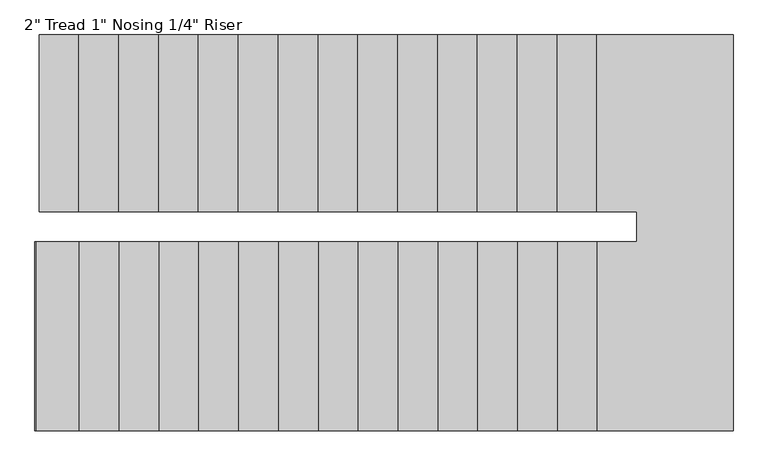
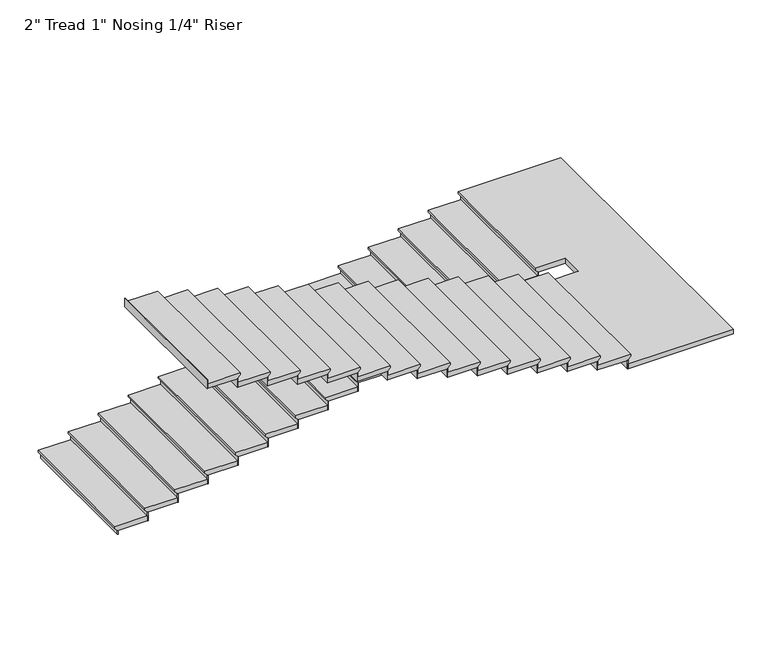
"""IFC4 building model written with IfcOpenShell, lengths in millimetres: stair flight geometry."""

from ifc_helpers import new_model, si_unit, origin, place, context, project, spatial, faceted_brep, source, transform, mapped, element, save


def stair_flight_f9fdc227(model_context):
    return source(origin(), model_context, "Body", "Brep", [
        faceted_brep([(-5254.0891351, 11154.2082924, 72.39), (-5254.0891351, 11154.2082924, 91.44), (-5254.0891351, 12506.0715905, 91.44), (-5254.0891351, 12506.0715905, 72.39), (-5228.6891351, 11154.2082924, 46.99), (-5228.6891351, 12506.0715905, 46.99), (-4923.8891351, 11154.2082924, 91.44), (-4923.8891351, 12506.0715905, 91.44), (-5228.6891351, 12506.0715905, 40.64), (-4923.8891351, 12506.0715905, 40.64), (-4923.8891351, 11154.2082924, 40.64), (-5228.6891351, 11154.2082924, 40.64)], [[[0, 1, 2, 3]], [[4, 0, 3, 5]], [[2, 1, 6, 7]], [[8, 9, 10, 11]], [[2, 7, 9, 8, 5, 3]], [[8, 11, 4, 5]], [[6, 1, 0, 4, 11, 10]], [[7, 6, 10, 9]]]),
        faceted_brep([(-5228.6891351, 11154.2082924, 40.64), (-5228.6891351, 11154.2082924, 0.0), (-5222.3391351, 11154.2082924, 0.0), (-5222.3391351, 11154.2082924, 40.64), (-5228.6891351, 12506.0715905, 40.64), (-5222.3391351, 12506.0715905, 40.64), (-5222.3391351, 12506.0715905, 0.0), (-5228.6891351, 12506.0715905, 0.0)], [[[0, 1, 2, 3]], [[4, 5, 6, 7]], [[1, 0, 4, 7]], [[2, 1, 7, 6]], [[3, 2, 6, 5]], [[0, 3, 5, 4]]]),
        faceted_brep([(-4923.8891351, 11154.2082924, 132.08), (-4923.8891351, 11154.2082924, 40.64), (-4917.5391351, 11154.2082924, 40.64), (-4917.5391351, 11154.2082924, 132.08), (-4923.8891351, 12506.0715905, 132.08), (-4917.5391351, 12506.0715905, 132.08), (-4917.5391351, 12506.0715905, 40.64), (-4923.8891351, 12506.0715905, 40.64)], [[[0, 1, 2, 3]], [[4, 5, 6, 7]], [[1, 0, 4, 7]], [[2, 1, 7, 6]], [[3, 2, 6, 5]], [[0, 3, 5, 4]]]),
        faceted_brep([(-4949.2891351, 12506.0715905, 182.88), (-4949.2891351, 11154.2082924, 182.88), (-4619.0891351, 11154.2082924, 182.88), (-4619.0891351, 12506.0715905, 182.88), (-4923.8891351, 12506.0715905, 132.08), (-4619.0891351, 12506.0715905, 132.08), (-4619.0891351, 11154.2082924, 132.08), (-4923.8891351, 11154.2082924, 132.08), (-4923.8891351, 12506.0715905, 138.43), (-4949.2891351, 12506.0715905, 163.83), (-4923.8891351, 11154.2082924, 138.43), (-4949.2891351, 11154.2082924, 163.83)], [[[0, 1, 2, 3]], [[4, 5, 6, 7]], [[0, 3, 5, 4, 8, 9]], [[4, 7, 10, 8]], [[2, 1, 11, 10, 7, 6]], [[3, 2, 6, 5]], [[11, 1, 0, 9]], [[10, 11, 9, 8]]]),
        faceted_brep([(-4619.0891351, 11154.2082924, 223.52), (-4619.0891351, 11154.2082924, 132.08), (-4612.7391351, 11154.2082924, 132.08), (-4612.7391351, 11154.2082924, 223.52), (-4619.0891351, 12506.0715905, 223.52), (-4612.7391351, 12506.0715905, 223.52), (-4612.7391351, 12506.0715905, 132.08), (-4619.0891351, 12506.0715905, 132.08)], [[[0, 1, 2, 3]], [[4, 5, 6, 7]], [[1, 0, 4, 7]], [[2, 1, 7, 6]], [[3, 2, 6, 5]], [[0, 3, 5, 4]]]),
        faceted_brep([(-4644.4891351, 12506.0715905, 274.32), (-4644.4891351, 11154.2082924, 274.32), (-4314.2891351, 11154.2082924, 274.32), (-4314.2891351, 12506.0715905, 274.32), (-4619.0891351, 12506.0715905, 223.52), (-4314.2891351, 12506.0715905, 223.52), (-4314.2891351, 11154.2082924, 223.52), (-4619.0891351, 11154.2082924, 223.52), (-4619.0891351, 12506.0715905, 229.87), (-4644.4891351, 12506.0715905, 255.27), (-4619.0891351, 11154.2082924, 229.87), (-4644.4891351, 11154.2082924, 255.27)], [[[0, 1, 2, 3]], [[4, 5, 6, 7]], [[0, 3, 5, 4, 8, 9]], [[4, 7, 10, 8]], [[2, 1, 11, 10, 7, 6]], [[3, 2, 6, 5]], [[11, 1, 0, 9]], [[10, 11, 9, 8]]]),
        faceted_brep([(-4314.2891351, 11154.2082924, 314.96), (-4314.2891351, 11154.2082924, 223.52), (-4307.9391351, 11154.2082924, 223.52), (-4307.9391351, 11154.2082924, 314.96), (-4314.2891351, 12506.0715905, 314.96), (-4307.9391351, 12506.0715905, 314.96), (-4307.9391351, 12506.0715905, 223.52), (-4314.2891351, 12506.0715905, 223.52)], [[[0, 1, 2, 3]], [[4, 5, 6, 7]], [[1, 0, 4, 7]], [[2, 1, 7, 6]], [[3, 2, 6, 5]], [[0, 3, 5, 4]]]),
        faceted_brep([(-4339.6891351, 12506.0715905, 365.76), (-4339.6891351, 11154.2082924, 365.76), (-4009.4891351, 11154.2082924, 365.76), (-4009.4891351, 12506.0715905, 365.76), (-4314.2891351, 12506.0715905, 314.96), (-4009.4891351, 12506.0715905, 314.96), (-4009.4891351, 11154.2082924, 314.96), (-4314.2891351, 11154.2082924, 314.96), (-4314.2891351, 12506.0715905, 321.31), (-4339.6891351, 12506.0715905, 346.71), (-4314.2891351, 11154.2082924, 321.31), (-4339.6891351, 11154.2082924, 346.71)], [[[0, 1, 2, 3]], [[4, 5, 6, 7]], [[0, 3, 5, 4, 8, 9]], [[4, 7, 10, 8]], [[2, 1, 11, 10, 7, 6]], [[3, 2, 6, 5]], [[11, 1, 0, 9]], [[10, 11, 9, 8]]]),
        faceted_brep([(-4009.4891351, 11154.2082924, 406.4), (-4009.4891351, 11154.2082924, 314.96), (-4003.1391351, 11154.2082924, 314.96), (-4003.1391351, 11154.2082924, 406.4), (-4009.4891351, 12506.0715905, 406.4), (-4003.1391351, 12506.0715905, 406.4), (-4003.1391351, 12506.0715905, 314.96), (-4009.4891351, 12506.0715905, 314.96)], [[[0, 1, 2, 3]], [[4, 5, 6, 7]], [[1, 0, 4, 7]], [[2, 1, 7, 6]], [[3, 2, 6, 5]], [[0, 3, 5, 4]]]),
        faceted_brep([(-4034.8891351, 12506.0715905, 457.2), (-4034.8891351, 11154.2082924, 457.2), (-3704.6891351, 11154.2082924, 457.2), (-3704.6891351, 12506.0715905, 457.2), (-4009.4891351, 12506.0715905, 406.4), (-3704.6891351, 12506.0715905, 406.4), (-3704.6891351, 11154.2082924, 406.4), (-4009.4891351, 11154.2082924, 406.4), (-4009.4891351, 12506.0715905, 412.75), (-4034.8891351, 12506.0715905, 438.15), (-4009.4891351, 11154.2082924, 412.75), (-4034.8891351, 11154.2082924, 438.15)], [[[0, 1, 2, 3]], [[4, 5, 6, 7]], [[0, 3, 5, 4, 8, 9]], [[4, 7, 10, 8]], [[2, 1, 11, 10, 7, 6]], [[3, 2, 6, 5]], [[11, 1, 0, 9]], [[10, 11, 9, 8]]]),
        faceted_brep([(-3704.6891351, 11154.2082924, 497.84), (-3704.6891351, 11154.2082924, 406.4), (-3698.3391351, 11154.2082924, 406.4), (-3698.3391351, 11154.2082924, 497.84), (-3704.6891351, 12506.0715905, 497.84), (-3698.3391351, 12506.0715905, 497.84), (-3698.3391351, 12506.0715905, 406.4), (-3704.6891351, 12506.0715905, 406.4)], [[[0, 1, 2, 3]], [[4, 5, 6, 7]], [[1, 0, 4, 7]], [[2, 1, 7, 6]], [[3, 2, 6, 5]], [[0, 3, 5, 4]]]),
        faceted_brep([(-3730.0891351, 12506.0715905, 548.64), (-3730.0891351, 11154.2082924, 548.64), (-3399.8891351, 11154.2082924, 548.64), (-3399.8891351, 12506.0715905, 548.64), (-3704.6891351, 12506.0715905, 497.84), (-3399.8891351, 12506.0715905, 497.84), (-3399.8891351, 11154.2082924, 497.84), (-3704.6891351, 11154.2082924, 497.84), (-3704.6891351, 12506.0715905, 504.19), (-3730.0891351, 12506.0715905, 529.59), (-3704.6891351, 11154.2082924, 504.19), (-3730.0891351, 11154.2082924, 529.59)], [[[0, 1, 2, 3]], [[4, 5, 6, 7]], [[0, 3, 5, 4, 8, 9]], [[4, 7, 10, 8]], [[2, 1, 11, 10, 7, 6]], [[3, 2, 6, 5]], [[11, 1, 0, 9]], [[10, 11, 9, 8]]]),
        faceted_brep([(-3399.8891351, 11154.2082924, 589.28), (-3399.8891351, 11154.2082924, 497.84), (-3393.5391351, 11154.2082924, 497.84), (-3393.5391351, 11154.2082924, 589.28), (-3399.8891351, 12506.0715905, 589.28), (-3393.5391351, 12506.0715905, 589.28), (-3393.5391351, 12506.0715905, 497.84), (-3399.8891351, 12506.0715905, 497.84)], [[[0, 1, 2, 3]], [[4, 5, 6, 7]], [[1, 0, 4, 7]], [[2, 1, 7, 6]], [[3, 2, 6, 5]], [[0, 3, 5, 4]]]),
        faceted_brep([(-3425.2891351, 12506.0715905, 640.08), (-3425.2891351, 11154.2082924, 640.08), (-3095.0891351, 11154.2082924, 640.08), (-3095.0891351, 12506.0715905, 640.08), (-3399.8891351, 12506.0715905, 589.28), (-3095.0891351, 12506.0715905, 589.28), (-3095.0891351, 11154.2082924, 589.28), (-3399.8891351, 11154.2082924, 589.28), (-3399.8891351, 12506.0715905, 595.63), (-3425.2891351, 12506.0715905, 621.03), (-3399.8891351, 11154.2082924, 595.63), (-3425.2891351, 11154.2082924, 621.03)], [[[0, 1, 2, 3]], [[4, 5, 6, 7]], [[0, 3, 5, 4, 8, 9]], [[4, 7, 10, 8]], [[2, 1, 11, 10, 7, 6]], [[3, 2, 6, 5]], [[11, 1, 0, 9]], [[10, 11, 9, 8]]]),
        faceted_brep([(-3095.0891351, 11154.2082924, 680.72), (-3095.0891351, 11154.2082924, 589.28), (-3088.7391351, 11154.2082924, 589.28), (-3088.7391351, 11154.2082924, 680.72), (-3095.0891351, 12506.0715905, 680.72), (-3088.7391351, 12506.0715905, 680.72), (-3088.7391351, 12506.0715905, 589.28), (-3095.0891351, 12506.0715905, 589.28)], [[[0, 1, 2, 3]], [[4, 5, 6, 7]], [[1, 0, 4, 7]], [[2, 1, 7, 6]], [[3, 2, 6, 5]], [[0, 3, 5, 4]]]),
        faceted_brep([(-3120.4891351, 12506.0715905, 731.52), (-3120.4891351, 11154.2082924, 731.52), (-2790.2891351, 11154.2082924, 731.52), (-2790.2891351, 12506.0715905, 731.52), (-3095.0891351, 12506.0715905, 680.72), (-2790.2891351, 12506.0715905, 680.72), (-2790.2891351, 11154.2082924, 680.72), (-3095.0891351, 11154.2082924, 680.72), (-3095.0891351, 12506.0715905, 687.07), (-3120.4891351, 12506.0715905, 712.47), (-3095.0891351, 11154.2082924, 687.07), (-3120.4891351, 11154.2082924, 712.47)], [[[0, 1, 2, 3]], [[4, 5, 6, 7]], [[0, 3, 5, 4, 8, 9]], [[4, 7, 10, 8]], [[2, 1, 11, 10, 7, 6]], [[3, 2, 6, 5]], [[11, 1, 0, 9]], [[10, 11, 9, 8]]]),
        faceted_brep([(-2790.2891351, 11154.2082924, 772.16), (-2790.2891351, 11154.2082924, 680.72), (-2783.9391351, 11154.2082924, 680.72), (-2783.9391351, 11154.2082924, 772.16), (-2790.2891351, 12506.0715905, 772.16), (-2783.9391351, 12506.0715905, 772.16), (-2783.9391351, 12506.0715905, 680.72), (-2790.2891351, 12506.0715905, 680.72)], [[[0, 1, 2, 3]], [[4, 5, 6, 7]], [[1, 0, 4, 7]], [[2, 1, 7, 6]], [[3, 2, 6, 5]], [[0, 3, 5, 4]]]),
        faceted_brep([(-2815.6891351, 12506.0715905, 822.96), (-2815.6891351, 11154.2082924, 822.96), (-2485.4891351, 11154.2082924, 822.96), (-2485.4891351, 12506.0715905, 822.96), (-2790.2891351, 12506.0715905, 772.16), (-2485.4891351, 12506.0715905, 772.16), (-2485.4891351, 11154.2082924, 772.16), (-2790.2891351, 11154.2082924, 772.16), (-2790.2891351, 12506.0715905, 778.51), (-2815.6891351, 12506.0715905, 803.91), (-2790.2891351, 11154.2082924, 778.51), (-2815.6891351, 11154.2082924, 803.91)], [[[0, 1, 2, 3]], [[4, 5, 6, 7]], [[0, 3, 5, 4, 8, 9]], [[4, 7, 10, 8]], [[2, 1, 11, 10, 7, 6]], [[3, 2, 6, 5]], [[11, 1, 0, 9]], [[10, 11, 9, 8]]]),
        faceted_brep([(-2485.4891351, 11154.2082924, 863.6), (-2485.4891351, 11154.2082924, 772.16), (-2479.1391351, 11154.2082924, 772.16), (-2479.1391351, 11154.2082924, 863.6), (-2485.4891351, 12506.0715905, 863.6), (-2479.1391351, 12506.0715905, 863.6), (-2479.1391351, 12506.0715905, 772.16), (-2485.4891351, 12506.0715905, 772.16)], [[[0, 1, 2, 3]], [[4, 5, 6, 7]], [[1, 0, 4, 7]], [[2, 1, 7, 6]], [[3, 2, 6, 5]], [[0, 3, 5, 4]]]),
        faceted_brep([(-2510.8891351, 12506.0715905, 914.4), (-2510.8891351, 11154.2082924, 914.4), (-2180.6891351, 11154.2082924, 914.4), (-2180.6891351, 12506.0715905, 914.4), (-2485.4891351, 12506.0715905, 863.6), (-2180.6891351, 12506.0715905, 863.6), (-2180.6891351, 11154.2082924, 863.6), (-2485.4891351, 11154.2082924, 863.6), (-2485.4891351, 12506.0715905, 869.95), (-2510.8891351, 12506.0715905, 895.35), (-2485.4891351, 11154.2082924, 869.95), (-2510.8891351, 11154.2082924, 895.35)], [[[0, 1, 2, 3]], [[4, 5, 6, 7]], [[0, 3, 5, 4, 8, 9]], [[4, 7, 10, 8]], [[2, 1, 11, 10, 7, 6]], [[3, 2, 6, 5]], [[11, 1, 0, 9]], [[10, 11, 9, 8]]]),
        faceted_brep([(-2180.6891351, 11154.2082924, 955.04), (-2180.6891351, 11154.2082924, 863.6), (-2174.3391351, 11154.2082924, 863.6), (-2174.3391351, 11154.2082924, 955.04), (-2180.6891351, 12506.0715905, 955.04), (-2174.3391351, 12506.0715905, 955.04), (-2174.3391351, 12506.0715905, 863.6), (-2180.6891351, 12506.0715905, 863.6)], [[[0, 1, 2, 3]], [[4, 5, 6, 7]], [[1, 0, 4, 7]], [[2, 1, 7, 6]], [[3, 2, 6, 5]], [[0, 3, 5, 4]]]),
        faceted_brep([(-2206.0891351, 12506.0715905, 1005.84), (-2206.0891351, 11154.2082924, 1005.84), (-1875.8891351, 11154.2082924, 1005.84), (-1875.8891351, 12506.0715905, 1005.84), (-2180.6891351, 12506.0715905, 955.04), (-1875.8891351, 12506.0715905, 955.04), (-1875.8891351, 11154.2082924, 955.04), (-2180.6891351, 11154.2082924, 955.04), (-2180.6891351, 12506.0715905, 961.39), (-2206.0891351, 12506.0715905, 986.79), (-2180.6891351, 11154.2082924, 961.39), (-2206.0891351, 11154.2082924, 986.79)], [[[0, 1, 2, 3]], [[4, 5, 6, 7]], [[0, 3, 5, 4, 8, 9]], [[4, 7, 10, 8]], [[2, 1, 11, 10, 7, 6]], [[3, 2, 6, 5]], [[11, 1, 0, 9]], [[10, 11, 9, 8]]]),
        faceted_brep([(-1875.8891351, 11154.2082924, 1046.48), (-1875.8891351, 11154.2082924, 955.04), (-1869.5391351, 11154.2082924, 955.04), (-1869.5391351, 11154.2082924, 1046.48), (-1875.8891351, 12506.0715905, 1046.48), (-1869.5391351, 12506.0715905, 1046.48), (-1869.5391351, 12506.0715905, 955.04), (-1875.8891351, 12506.0715905, 955.04)], [[[0, 1, 2, 3]], [[4, 5, 6, 7]], [[1, 0, 4, 7]], [[2, 1, 7, 6]], [[3, 2, 6, 5]], [[0, 3, 5, 4]]]),
        faceted_brep([(-1901.2891351, 12506.0715905, 1097.28), (-1901.2891351, 11154.2082924, 1097.28), (-1571.0891351, 11154.2082924, 1097.28), (-1571.0891351, 12506.0715905, 1097.28), (-1875.8891351, 12506.0715905, 1046.48), (-1571.0891351, 12506.0715905, 1046.48), (-1571.0891351, 11154.2082924, 1046.48), (-1875.8891351, 11154.2082924, 1046.48), (-1875.8891351, 12506.0715905, 1052.83), (-1901.2891351, 12506.0715905, 1078.23), (-1875.8891351, 11154.2082924, 1052.83), (-1901.2891351, 11154.2082924, 1078.23)], [[[0, 1, 2, 3]], [[4, 5, 6, 7]], [[0, 3, 5, 4, 8, 9]], [[4, 7, 10, 8]], [[2, 1, 11, 10, 7, 6]], [[3, 2, 6, 5]], [[11, 1, 0, 9]], [[10, 11, 9, 8]]]),
        faceted_brep([(-1571.0891351, 11154.2082924, 1137.92), (-1571.0891351, 11154.2082924, 1046.48), (-1564.7391351, 11154.2082924, 1046.48), (-1564.7391351, 11154.2082924, 1137.92), (-1571.0891351, 12506.0715905, 1137.92), (-1564.7391351, 12506.0715905, 1137.92), (-1564.7391351, 12506.0715905, 1046.48), (-1571.0891351, 12506.0715905, 1046.48)], [[[0, 1, 2, 3]], [[4, 5, 6, 7]], [[1, 0, 4, 7]], [[2, 1, 7, 6]], [[3, 2, 6, 5]], [[0, 3, 5, 4]]]),
        faceted_brep([(-1596.4891351, 12506.0715905, 1188.72), (-1596.4891351, 11154.2082924, 1188.72), (-1266.2891351, 11154.2082924, 1188.72), (-1266.2891351, 12506.0715905, 1188.72), (-1571.0891351, 12506.0715905, 1137.92), (-1266.2891351, 12506.0715905, 1137.92), (-1266.2891351, 11154.2082924, 1137.92), (-1571.0891351, 11154.2082924, 1137.92), (-1571.0891351, 12506.0715905, 1144.27), (-1596.4891351, 12506.0715905, 1169.67), (-1571.0891351, 11154.2082924, 1144.27), (-1596.4891351, 11154.2082924, 1169.67)], [[[0, 1, 2, 3]], [[4, 5, 6, 7]], [[0, 3, 5, 4, 8, 9]], [[4, 7, 10, 8]], [[2, 1, 11, 10, 7, 6]], [[3, 2, 6, 5]], [[11, 1, 0, 9]], [[10, 11, 9, 8]]]),
        faceted_brep([(-1266.2891351, 11154.2082924, 1229.36), (-1266.2891351, 11154.2082924, 1137.92), (-1259.9391351, 11154.2082924, 1137.92), (-1259.9391351, 11154.2082924, 1229.36), (-1266.2891351, 12506.0715905, 1229.36), (-1259.9391351, 12506.0715905, 1229.36), (-1259.9391351, 12506.0715905, 1137.92), (-1266.2891351, 12506.0715905, 1137.92)], [[[0, 1, 2, 3]], [[4, 5, 6, 7]], [[1, 0, 4, 7]], [[2, 1, 7, 6]], [[3, 2, 6, 5]], [[0, 3, 5, 4]]]),
        faceted_brep([(-1291.6891351, 12506.0715905, 1280.16), (-1291.6891351, 11154.2082924, 1280.16), (-961.4891351, 11154.2082924, 1280.16), (-961.4891351, 12506.0715905, 1280.16), (-1266.2891351, 12506.0715905, 1229.36), (-961.4891351, 12506.0715905, 1229.36), (-961.4891351, 11154.2082924, 1229.36), (-1266.2891351, 11154.2082924, 1229.36), (-1266.2891351, 12506.0715905, 1235.71), (-1291.6891351, 12506.0715905, 1261.11), (-1266.2891351, 11154.2082924, 1235.71), (-1291.6891351, 11154.2082924, 1261.11)], [[[0, 1, 2, 3]], [[4, 5, 6, 7]], [[0, 3, 5, 4, 8, 9]], [[4, 7, 10, 8]], [[2, 1, 11, 10, 7, 6]], [[3, 2, 6, 5]], [[11, 1, 0, 9]], [[10, 11, 9, 8]]]),
        faceted_brep([(-961.4891351, 11154.2082924, 1320.8), (-961.4891351, 11154.2082924, 1229.36), (-955.1391351, 11154.2082924, 1229.36), (-955.1391351, 11154.2082924, 1320.8), (-961.4891351, 12506.0715905, 1320.8), (-955.1391351, 12506.0715905, 1320.8), (-955.1391351, 12506.0715905, 1229.36), (-961.4891351, 12506.0715905, 1229.36)], [[[0, 1, 2, 3]], [[4, 5, 6, 7]], [[1, 0, 4, 7]], [[2, 1, 7, 6]], [[3, 2, 6, 5]], [[0, 3, 5, 4]]]),
        faceted_brep([(-1012.2891351, 9478.4949943, 1371.6), (54.5108649, 9478.4949943, 1371.6), (54.5108649, 12506.0715905, 1371.6), (-986.8891351, 12506.0715905, 1371.6), (-986.8891351, 11154.2082924, 1371.6), (-682.0891351, 11154.2082924, 1371.6), (-682.0891351, 10925.6082924, 1371.6), (-1012.2891351, 10925.6082924, 1371.6), (54.5108649, 9478.4949943, 1320.8), (-1012.2891351, 9478.4949943, 1320.8), (-1012.2891351, 10925.6082924, 1320.8), (-682.0891351, 10925.6082924, 1320.8), (-682.0891351, 11154.2082924, 1320.8), (-961.4891351, 11154.2082924, 1320.8), (-961.4891351, 12506.0715905, 1320.8), (54.5108649, 12506.0715905, 1320.8), (-961.4891351, 12506.0715905, 1327.15), (-986.8891351, 12506.0715905, 1352.55), (-961.4891351, 11154.2082924, 1327.15), (-986.8891351, 11154.2082924, 1352.55)], [[[0, 1, 2, 3, 4, 5, 6, 7]], [[8, 9, 10, 11, 12, 13, 14, 15]], [[1, 0, 9, 8]], [[2, 1, 8, 15]], [[3, 2, 15, 14, 16, 17]], [[14, 13, 18, 16]], [[5, 4, 19, 18, 13, 12]], [[6, 5, 12, 11]], [[7, 6, 11, 10]], [[0, 7, 10, 9]], [[19, 4, 3, 17]], [[18, 19, 17, 16]]]),
        faceted_brep([(-1012.2891351, 10925.6082924, 1412.24), (-1012.2891351, 10925.6082924, 1320.8), (-1018.6391351, 10925.6082924, 1320.8), (-1018.6391351, 10925.6082924, 1412.24), (-1012.2891351, 9478.4949943, 1412.24), (-1018.6391351, 9478.4949943, 1412.24), (-1018.6391351, 9478.4949943, 1320.8), (-1012.2891351, 9478.4949943, 1320.8)], [[[0, 1, 2, 3]], [[4, 5, 6, 7]], [[1, 0, 4, 7]], [[2, 1, 7, 6]], [[3, 2, 6, 5]], [[0, 3, 5, 4]]]),
        faceted_brep([(-986.8891351, 9478.4949943, 1463.04), (-986.8891351, 10925.6082924, 1463.04), (-1317.0891351, 10925.6082924, 1463.04), (-1317.0891351, 9478.4949943, 1463.04), (-1012.2891351, 9478.4949943, 1412.24), (-1317.0891351, 9478.4949943, 1412.24), (-1317.0891351, 10925.6082924, 1412.24), (-1012.2891351, 10925.6082924, 1412.24), (-1012.2891351, 9478.4949943, 1418.59), (-986.8891351, 9478.4949943, 1443.99), (-1012.2891351, 10925.6082924, 1418.59), (-986.8891351, 10925.6082924, 1443.99)], [[[0, 1, 2, 3]], [[4, 5, 6, 7]], [[0, 3, 5, 4, 8, 9]], [[4, 7, 10, 8]], [[2, 1, 11, 10, 7, 6]], [[3, 2, 6, 5]], [[11, 1, 0, 9]], [[10, 11, 9, 8]]]),
        faceted_brep([(-1317.0891351, 10925.6082924, 1503.68), (-1317.0891351, 10925.6082924, 1412.24), (-1323.4391351, 10925.6082924, 1412.24), (-1323.4391351, 10925.6082924, 1503.68), (-1317.0891351, 9478.4949943, 1503.68), (-1323.4391351, 9478.4949943, 1503.68), (-1323.4391351, 9478.4949943, 1412.24), (-1317.0891351, 9478.4949943, 1412.24)], [[[0, 1, 2, 3]], [[4, 5, 6, 7]], [[1, 0, 4, 7]], [[2, 1, 7, 6]], [[3, 2, 6, 5]], [[0, 3, 5, 4]]]),
        faceted_brep([(-1291.6891351, 9478.4949943, 1554.48), (-1291.6891351, 10925.6082924, 1554.48), (-1621.8891351, 10925.6082924, 1554.48), (-1621.8891351, 9478.4949943, 1554.48), (-1317.0891351, 9478.4949943, 1503.68), (-1621.8891351, 9478.4949943, 1503.68), (-1621.8891351, 10925.6082924, 1503.68), (-1317.0891351, 10925.6082924, 1503.68), (-1317.0891351, 9478.4949943, 1510.03), (-1291.6891351, 9478.4949943, 1535.43), (-1317.0891351, 10925.6082924, 1510.03), (-1291.6891351, 10925.6082924, 1535.43)], [[[0, 1, 2, 3]], [[4, 5, 6, 7]], [[0, 3, 5, 4, 8, 9]], [[4, 7, 10, 8]], [[2, 1, 11, 10, 7, 6]], [[3, 2, 6, 5]], [[11, 1, 0, 9]], [[10, 11, 9, 8]]]),
        faceted_brep([(-1621.8891351, 10925.6082924, 1595.12), (-1621.8891351, 10925.6082924, 1503.68), (-1628.2391351, 10925.6082924, 1503.68), (-1628.2391351, 10925.6082924, 1595.12), (-1621.8891351, 9478.4949943, 1595.12), (-1628.2391351, 9478.4949943, 1595.12), (-1628.2391351, 9478.4949943, 1503.68), (-1621.8891351, 9478.4949943, 1503.68)], [[[0, 1, 2, 3]], [[4, 5, 6, 7]], [[1, 0, 4, 7]], [[2, 1, 7, 6]], [[3, 2, 6, 5]], [[0, 3, 5, 4]]]),
        faceted_brep([(-1596.4891351, 9478.4949943, 1645.92), (-1596.4891351, 10925.6082924, 1645.92), (-1926.6891351, 10925.6082924, 1645.92), (-1926.6891351, 9478.4949943, 1645.92), (-1621.8891351, 9478.4949943, 1595.12), (-1926.6891351, 9478.4949943, 1595.12), (-1926.6891351, 10925.6082924, 1595.12), (-1621.8891351, 10925.6082924, 1595.12), (-1621.8891351, 9478.4949943, 1601.47), (-1596.4891351, 9478.4949943, 1626.87), (-1621.8891351, 10925.6082924, 1601.47), (-1596.4891351, 10925.6082924, 1626.87)], [[[0, 1, 2, 3]], [[4, 5, 6, 7]], [[0, 3, 5, 4, 8, 9]], [[4, 7, 10, 8]], [[2, 1, 11, 10, 7, 6]], [[3, 2, 6, 5]], [[11, 1, 0, 9]], [[10, 11, 9, 8]]]),
        faceted_brep([(-1926.6891351, 10925.6082924, 1686.56), (-1926.6891351, 10925.6082924, 1595.12), (-1933.0391351, 10925.6082924, 1595.12), (-1933.0391351, 10925.6082924, 1686.56), (-1926.6891351, 9478.4949943, 1686.56), (-1933.0391351, 9478.4949943, 1686.56), (-1933.0391351, 9478.4949943, 1595.12), (-1926.6891351, 9478.4949943, 1595.12)], [[[0, 1, 2, 3]], [[4, 5, 6, 7]], [[1, 0, 4, 7]], [[2, 1, 7, 6]], [[3, 2, 6, 5]], [[0, 3, 5, 4]]]),
        faceted_brep([(-1901.2891351, 9478.4949943, 1737.36), (-1901.2891351, 10925.6082924, 1737.36), (-2231.4891351, 10925.6082924, 1737.36), (-2231.4891351, 9478.4949943, 1737.36), (-1926.6891351, 9478.4949943, 1686.56), (-2231.4891351, 9478.4949943, 1686.56), (-2231.4891351, 10925.6082924, 1686.56), (-1926.6891351, 10925.6082924, 1686.56), (-1926.6891351, 9478.4949943, 1692.91), (-1901.2891351, 9478.4949943, 1718.31), (-1926.6891351, 10925.6082924, 1692.91), (-1901.2891351, 10925.6082924, 1718.31)], [[[0, 1, 2, 3]], [[4, 5, 6, 7]], [[0, 3, 5, 4, 8, 9]], [[4, 7, 10, 8]], [[2, 1, 11, 10, 7, 6]], [[3, 2, 6, 5]], [[11, 1, 0, 9]], [[10, 11, 9, 8]]]),
        faceted_brep([(-2231.4891351, 10925.6082924, 1778.0), (-2231.4891351, 10925.6082924, 1686.56), (-2237.8391351, 10925.6082924, 1686.56), (-2237.8391351, 10925.6082924, 1778.0), (-2231.4891351, 9478.4949943, 1778.0), (-2237.8391351, 9478.4949943, 1778.0), (-2237.8391351, 9478.4949943, 1686.56), (-2231.4891351, 9478.4949943, 1686.56)], [[[0, 1, 2, 3]], [[4, 5, 6, 7]], [[1, 0, 4, 7]], [[2, 1, 7, 6]], [[3, 2, 6, 5]], [[0, 3, 5, 4]]]),
        faceted_brep([(-2206.0891351, 9478.4949943, 1828.8), (-2206.0891351, 10925.6082924, 1828.8), (-2536.2891351, 10925.6082924, 1828.8), (-2536.2891351, 9478.4949943, 1828.8), (-2231.4891351, 9478.4949943, 1778.0), (-2536.2891351, 9478.4949943, 1778.0), (-2536.2891351, 10925.6082924, 1778.0), (-2231.4891351, 10925.6082924, 1778.0), (-2231.4891351, 9478.4949943, 1784.35), (-2206.0891351, 9478.4949943, 1809.75), (-2231.4891351, 10925.6082924, 1784.35), (-2206.0891351, 10925.6082924, 1809.75)], [[[0, 1, 2, 3]], [[4, 5, 6, 7]], [[0, 3, 5, 4, 8, 9]], [[4, 7, 10, 8]], [[2, 1, 11, 10, 7, 6]], [[3, 2, 6, 5]], [[11, 1, 0, 9]], [[10, 11, 9, 8]]]),
        faceted_brep([(-2536.2891351, 10925.6082924, 1869.44), (-2536.2891351, 10925.6082924, 1778.0), (-2542.6391351, 10925.6082924, 1778.0), (-2542.6391351, 10925.6082924, 1869.44), (-2536.2891351, 9478.4949943, 1869.44), (-2542.6391351, 9478.4949943, 1869.44), (-2542.6391351, 9478.4949943, 1778.0), (-2536.2891351, 9478.4949943, 1778.0)], [[[0, 1, 2, 3]], [[4, 5, 6, 7]], [[1, 0, 4, 7]], [[2, 1, 7, 6]], [[3, 2, 6, 5]], [[0, 3, 5, 4]]]),
        faceted_brep([(-2510.8891351, 9478.4949943, 1920.24), (-2510.8891351, 10925.6082924, 1920.24), (-2841.0891351, 10925.6082924, 1920.24), (-2841.0891351, 9478.4949943, 1920.24), (-2536.2891351, 9478.4949943, 1869.44), (-2841.0891351, 9478.4949943, 1869.44), (-2841.0891351, 10925.6082924, 1869.44), (-2536.2891351, 10925.6082924, 1869.44), (-2536.2891351, 9478.4949943, 1875.79), (-2510.8891351, 9478.4949943, 1901.19), (-2536.2891351, 10925.6082924, 1875.79), (-2510.8891351, 10925.6082924, 1901.19)], [[[0, 1, 2, 3]], [[4, 5, 6, 7]], [[0, 3, 5, 4, 8, 9]], [[4, 7, 10, 8]], [[2, 1, 11, 10, 7, 6]], [[3, 2, 6, 5]], [[11, 1, 0, 9]], [[10, 11, 9, 8]]]),
        faceted_brep([(-2841.0891351, 10925.6082924, 1960.88), (-2841.0891351, 10925.6082924, 1869.44), (-2847.4391351, 10925.6082924, 1869.44), (-2847.4391351, 10925.6082924, 1960.88), (-2841.0891351, 9478.4949943, 1960.88), (-2847.4391351, 9478.4949943, 1960.88), (-2847.4391351, 9478.4949943, 1869.44), (-2841.0891351, 9478.4949943, 1869.44)], [[[0, 1, 2, 3]], [[4, 5, 6, 7]], [[1, 0, 4, 7]], [[2, 1, 7, 6]], [[3, 2, 6, 5]], [[0, 3, 5, 4]]]),
        faceted_brep([(-2815.6891351, 9478.4949943, 2011.68), (-2815.6891351, 10925.6082924, 2011.68), (-3145.8891351, 10925.6082924, 2011.68), (-3145.8891351, 9478.4949943, 2011.68), (-2841.0891351, 9478.4949943, 1960.88), (-3145.8891351, 9478.4949943, 1960.88), (-3145.8891351, 10925.6082924, 1960.88), (-2841.0891351, 10925.6082924, 1960.88), (-2841.0891351, 9478.4949943, 1967.23), (-2815.6891351, 9478.4949943, 1992.63), (-2841.0891351, 10925.6082924, 1967.23), (-2815.6891351, 10925.6082924, 1992.63)], [[[0, 1, 2, 3]], [[4, 5, 6, 7]], [[0, 3, 5, 4, 8, 9]], [[4, 7, 10, 8]], [[2, 1, 11, 10, 7, 6]], [[3, 2, 6, 5]], [[11, 1, 0, 9]], [[10, 11, 9, 8]]]),
        faceted_brep([(-3145.8891351, 10925.6082924, 2052.32), (-3145.8891351, 10925.6082924, 1960.88), (-3152.2391351, 10925.6082924, 1960.88), (-3152.2391351, 10925.6082924, 2052.32), (-3145.8891351, 9478.4949943, 2052.32), (-3152.2391351, 9478.4949943, 2052.32), (-3152.2391351, 9478.4949943, 1960.88), (-3145.8891351, 9478.4949943, 1960.88)], [[[0, 1, 2, 3]], [[4, 5, 6, 7]], [[1, 0, 4, 7]], [[2, 1, 7, 6]], [[3, 2, 6, 5]], [[0, 3, 5, 4]]]),
        faceted_brep([(-3120.4891351, 9478.4949943, 2103.12), (-3120.4891351, 10925.6082924, 2103.12), (-3450.6891351, 10925.6082924, 2103.12), (-3450.6891351, 9478.4949943, 2103.12), (-3145.8891351, 9478.4949943, 2052.32), (-3450.6891351, 9478.4949943, 2052.32), (-3450.6891351, 10925.6082924, 2052.32), (-3145.8891351, 10925.6082924, 2052.32), (-3145.8891351, 9478.4949943, 2058.67), (-3120.4891351, 9478.4949943, 2084.07), (-3145.8891351, 10925.6082924, 2058.67), (-3120.4891351, 10925.6082924, 2084.07)], [[[0, 1, 2, 3]], [[4, 5, 6, 7]], [[0, 3, 5, 4, 8, 9]], [[4, 7, 10, 8]], [[2, 1, 11, 10, 7, 6]], [[3, 2, 6, 5]], [[11, 1, 0, 9]], [[10, 11, 9, 8]]]),
        faceted_brep([(-3450.6891351, 10925.6082924, 2143.76), (-3450.6891351, 10925.6082924, 2052.32), (-3457.0391351, 10925.6082924, 2052.32), (-3457.0391351, 10925.6082924, 2143.76), (-3450.6891351, 9478.4949943, 2143.76), (-3457.0391351, 9478.4949943, 2143.76), (-3457.0391351, 9478.4949943, 2052.32), (-3450.6891351, 9478.4949943, 2052.32)], [[[0, 1, 2, 3]], [[4, 5, 6, 7]], [[1, 0, 4, 7]], [[2, 1, 7, 6]], [[3, 2, 6, 5]], [[0, 3, 5, 4]]]),
        faceted_brep([(-3425.2891351, 9478.4949943, 2194.56), (-3425.2891351, 10925.6082924, 2194.56), (-3755.4891351, 10925.6082924, 2194.56), (-3755.4891351, 9478.4949943, 2194.56), (-3450.6891351, 9478.4949943, 2143.76), (-3755.4891351, 9478.4949943, 2143.76), (-3755.4891351, 10925.6082924, 2143.76), (-3450.6891351, 10925.6082924, 2143.76), (-3450.6891351, 9478.4949943, 2150.11), (-3425.2891351, 9478.4949943, 2175.51), (-3450.6891351, 10925.6082924, 2150.11), (-3425.2891351, 10925.6082924, 2175.51)], [[[0, 1, 2, 3]], [[4, 5, 6, 7]], [[0, 3, 5, 4, 8, 9]], [[4, 7, 10, 8]], [[2, 1, 11, 10, 7, 6]], [[3, 2, 6, 5]], [[11, 1, 0, 9]], [[10, 11, 9, 8]]]),
        faceted_brep([(-3755.4891351, 10925.6082924, 2235.2), (-3755.4891351, 10925.6082924, 2143.76), (-3761.8391351, 10925.6082924, 2143.76), (-3761.8391351, 10925.6082924, 2235.2), (-3755.4891351, 9478.4949943, 2235.2), (-3761.8391351, 9478.4949943, 2235.2), (-3761.8391351, 9478.4949943, 2143.76), (-3755.4891351, 9478.4949943, 2143.76)], [[[0, 1, 2, 3]], [[4, 5, 6, 7]], [[1, 0, 4, 7]], [[2, 1, 7, 6]], [[3, 2, 6, 5]], [[0, 3, 5, 4]]]),
        faceted_brep([(-3730.0891351, 9478.4949943, 2286.0), (-3730.0891351, 10925.6082924, 2286.0), (-4060.2891351, 10925.6082924, 2286.0), (-4060.2891351, 9478.4949943, 2286.0), (-3755.4891351, 9478.4949943, 2235.2), (-4060.2891351, 9478.4949943, 2235.2), (-4060.2891351, 10925.6082924, 2235.2), (-3755.4891351, 10925.6082924, 2235.2), (-3755.4891351, 9478.4949943, 2241.55), (-3730.0891351, 9478.4949943, 2266.95), (-3755.4891351, 10925.6082924, 2241.55), (-3730.0891351, 10925.6082924, 2266.95)], [[[0, 1, 2, 3]], [[4, 5, 6, 7]], [[0, 3, 5, 4, 8, 9]], [[4, 7, 10, 8]], [[2, 1, 11, 10, 7, 6]], [[3, 2, 6, 5]], [[11, 1, 0, 9]], [[10, 11, 9, 8]]]),
        faceted_brep([(-4060.2891351, 10925.6082924, 2326.64), (-4060.2891351, 10925.6082924, 2235.2), (-4066.6391351, 10925.6082924, 2235.2), (-4066.6391351, 10925.6082924, 2326.64), (-4060.2891351, 9478.4949943, 2326.64), (-4066.6391351, 9478.4949943, 2326.64), (-4066.6391351, 9478.4949943, 2235.2), (-4060.2891351, 9478.4949943, 2235.2)], [[[0, 1, 2, 3]], [[4, 5, 6, 7]], [[1, 0, 4, 7]], [[2, 1, 7, 6]], [[3, 2, 6, 5]], [[0, 3, 5, 4]]]),
        faceted_brep([(-4034.8891351, 9478.4949943, 2377.44), (-4034.8891351, 10925.6082924, 2377.44), (-4365.0891351, 10925.6082924, 2377.44), (-4365.0891351, 9478.4949943, 2377.44), (-4060.2891351, 9478.4949943, 2326.64), (-4365.0891351, 9478.4949943, 2326.64), (-4365.0891351, 10925.6082924, 2326.64), (-4060.2891351, 10925.6082924, 2326.64), (-4060.2891351, 9478.4949943, 2332.99), (-4034.8891351, 9478.4949943, 2358.39), (-4060.2891351, 10925.6082924, 2332.99), (-4034.8891351, 10925.6082924, 2358.39)], [[[0, 1, 2, 3]], [[4, 5, 6, 7]], [[0, 3, 5, 4, 8, 9]], [[4, 7, 10, 8]], [[2, 1, 11, 10, 7, 6]], [[3, 2, 6, 5]], [[11, 1, 0, 9]], [[10, 11, 9, 8]]]),
        faceted_brep([(-4365.0891351, 10925.6082924, 2418.08), (-4365.0891351, 10925.6082924, 2326.64), (-4371.4391351, 10925.6082924, 2326.64), (-4371.4391351, 10925.6082924, 2418.08), (-4365.0891351, 9478.4949943, 2418.08), (-4371.4391351, 9478.4949943, 2418.08), (-4371.4391351, 9478.4949943, 2326.64), (-4365.0891351, 9478.4949943, 2326.64)], [[[0, 1, 2, 3]], [[4, 5, 6, 7]], [[1, 0, 4, 7]], [[2, 1, 7, 6]], [[3, 2, 6, 5]], [[0, 3, 5, 4]]]),
        faceted_brep([(-4339.6891351, 9478.4949943, 2468.88), (-4339.6891351, 10925.6082924, 2468.88), (-4669.8891351, 10925.6082924, 2468.88), (-4669.8891351, 9478.4949943, 2468.88), (-4365.0891351, 9478.4949943, 2418.08), (-4669.8891351, 9478.4949943, 2418.08), (-4669.8891351, 10925.6082924, 2418.08), (-4365.0891351, 10925.6082924, 2418.08), (-4365.0891351, 9478.4949943, 2424.43), (-4339.6891351, 9478.4949943, 2449.83), (-4365.0891351, 10925.6082924, 2424.43), (-4339.6891351, 10925.6082924, 2449.83)], [[[0, 1, 2, 3]], [[4, 5, 6, 7]], [[0, 3, 5, 4, 8, 9]], [[4, 7, 10, 8]], [[2, 1, 11, 10, 7, 6]], [[3, 2, 6, 5]], [[11, 1, 0, 9]], [[10, 11, 9, 8]]]),
        faceted_brep([(-4669.8891351, 10925.6082924, 2509.52), (-4669.8891351, 10925.6082924, 2418.08), (-4676.2391351, 10925.6082924, 2418.08), (-4676.2391351, 10925.6082924, 2509.52), (-4669.8891351, 9478.4949943, 2509.52), (-4676.2391351, 9478.4949943, 2509.52), (-4676.2391351, 9478.4949943, 2418.08), (-4669.8891351, 9478.4949943, 2418.08)], [[[0, 1, 2, 3]], [[4, 5, 6, 7]], [[1, 0, 4, 7]], [[2, 1, 7, 6]], [[3, 2, 6, 5]], [[0, 3, 5, 4]]]),
        faceted_brep([(-4644.4891351, 9478.4949943, 2560.32), (-4644.4891351, 10925.6082924, 2560.32), (-4974.6891351, 10925.6082924, 2560.32), (-4974.6891351, 9478.4949943, 2560.32), (-4669.8891351, 9478.4949943, 2509.52), (-4974.6891351, 9478.4949943, 2509.52), (-4974.6891351, 10925.6082924, 2509.52), (-4669.8891351, 10925.6082924, 2509.52), (-4669.8891351, 9478.4949943, 2515.87), (-4644.4891351, 9478.4949943, 2541.27), (-4669.8891351, 10925.6082924, 2515.87), (-4644.4891351, 10925.6082924, 2541.27)], [[[0, 1, 2, 3]], [[4, 5, 6, 7]], [[0, 3, 5, 4, 8, 9]], [[4, 7, 10, 8]], [[2, 1, 11, 10, 7, 6]], [[3, 2, 6, 5]], [[11, 1, 0, 9]], [[10, 11, 9, 8]]]),
        faceted_brep([(-4974.6891351, 10925.6082924, 2600.96), (-4974.6891351, 10925.6082924, 2509.52), (-4981.0391351, 10925.6082924, 2509.52), (-4981.0391351, 10925.6082924, 2600.96), (-4974.6891351, 9478.4949943, 2600.96), (-4981.0391351, 9478.4949943, 2600.96), (-4981.0391351, 9478.4949943, 2509.52), (-4974.6891351, 9478.4949943, 2509.52)], [[[0, 1, 2, 3]], [[4, 5, 6, 7]], [[1, 0, 4, 7]], [[2, 1, 7, 6]], [[3, 2, 6, 5]], [[0, 3, 5, 4]]]),
        faceted_brep([(-5279.4891351, 10925.6082924, 2692.4), (-5279.4891351, 10925.6082924, 2600.96), (-5285.8391351, 10925.6082924, 2600.96), (-5285.8391351, 10925.6082924, 2692.4), (-5279.4891351, 9478.4949943, 2692.4), (-5285.8391351, 9478.4949943, 2692.4), (-5285.8391351, 9478.4949943, 2600.96), (-5279.4891351, 9478.4949943, 2600.96)], [[[0, 1, 2, 3]], [[4, 5, 6, 7]], [[1, 0, 4, 7]], [[2, 1, 7, 6]], [[3, 2, 6, 5]], [[0, 3, 5, 4]]]),
        faceted_brep([(-4949.2891351, 9478.4949943, 2651.76), (-4949.2891351, 10925.6082924, 2651.76), (-5279.4891351, 10925.6082924, 2651.76), (-5279.4891351, 9478.4949943, 2651.76), (-4974.6891351, 9478.4949943, 2600.96), (-5279.4891351, 9478.4949943, 2600.96), (-5279.4891351, 10925.6082924, 2600.96), (-4974.6891351, 10925.6082924, 2600.96), (-4974.6891351, 9478.4949943, 2607.31), (-4949.2891351, 9478.4949943, 2632.71), (-4974.6891351, 10925.6082924, 2607.31), (-4949.2891351, 10925.6082924, 2632.71)], [[[0, 1, 2, 3]], [[4, 5, 6, 7]], [[0, 3, 5, 4, 8, 9]], [[4, 7, 10, 8]], [[2, 1, 11, 10, 7, 6]], [[3, 2, 6, 5]], [[11, 1, 0, 9]], [[10, 11, 9, 8]]]),
    ])


if __name__ == "__main__":
    model = new_model("IFC4")
    model_context = context("Model", 3, world=origin())
    ifc_project = project(units=[si_unit("LENGTHUNIT", "METRE", prefix="MILLI")], contexts=[model_context])
    site = spatial("IfcSite", under=ifc_project)
    building = spatial("IfcBuilding", under=site)
    placement = place(None, origin())
    stair_flight_shape = stair_flight_f9fdc227(model_context)
    element("IfcStairFlight", 1, ObjectType="2\" Tread 1\" Nosing 1/4\" Riser", at=placement, inside=building, context=model_context, shape_type="MappedRepresentation", body=[
        mapped(stair_flight_shape, transform((0.0, 0.0, 0.0), x_axis=(1.0, 0.0, 0.0), y_axis=(0.0, 1.0, 0.0), z_axis=(0.0, 0.0, 1.0))),
    ])
    save(model, "model.ifc")
